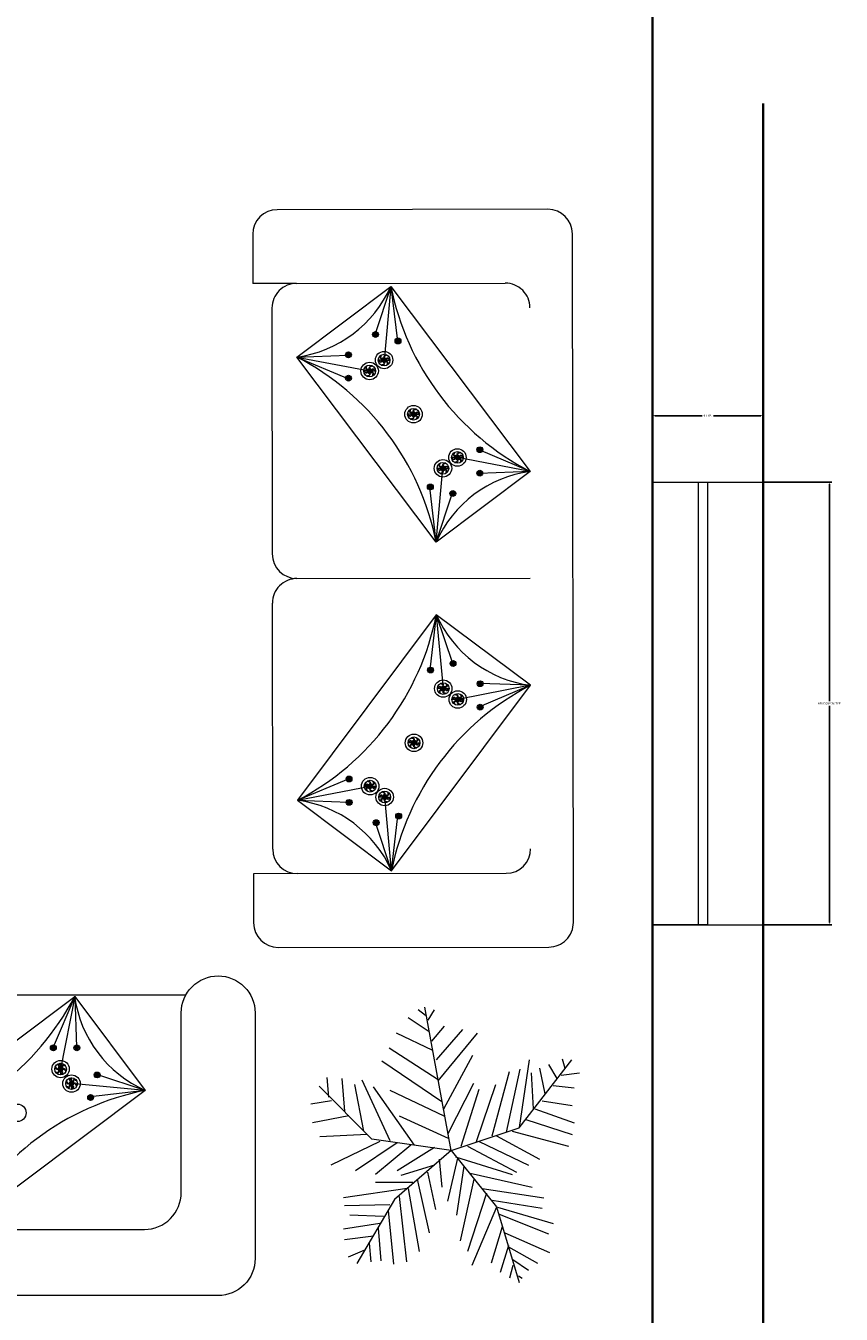
# Model space of a CAD drawing. Units: inches. Extents: x -61 to 1599, y -1316 to 257.
# Tile 199 of 204: x 1463 to 1529, y -166 to -61. Entities that reach past the tile are written whole.
import ezdxf

# ---------------------------------------------------------------- set-up
doc = ezdxf.new("R2010")
doc.units = ezdxf.units.IN
doc.header["$MEASUREMENT"] = 0
for name, color, linetype, lineweight in [('A-ANNO-DIMS', 2, 'Continuous', 18), ('FURNITURE', 83, 'Continuous', 18), ('WALLS', 4, 'Continuous', 35), ('WINDOWS', 220, 'Continuous', 18)]:
    doc.layers.add(name, color=color, linetype=linetype, lineweight=lineweight)
doc.layers.add('FUR', color=83, linetype='Continuous')
doc.styles.get("Standard").update_dxf_attribs({"font": 'arial.ttf'})
doc.dimstyles.get("Standard").update_dxf_attribs({"dimtxt": 0.18, "dimasz": 0.18, "dimexe": 0.18, "dimexo": 0.0625, "dimgap": 0.09, "dimtad": 0, "dimtih": 1, "dimtoh": 1, "dimdec": 0, "dimzin": 0, "dimdsep": 46, "dimlunit": 3, "dimtxsty": 'Standard', "dimcen": 0.09, "dimadec": 0, "dimazin": 0, "dimtfac": 1, "dimtdec": 0, "dimtofl": 0, "dimtmove": 0, "dimatfit": 3, "dimfxl": 1, "dimtolj": 1, "dimtzin": 0, "dimarcsym": 0})

# ---------------------------------------------------------------- blocks, each defined once
blk = doc.blocks.new('*U427')
at = {"layer": 'FUR'}
blk.add_open_spline([(0.01, 0.24), (-0.09, 0.14), (-0.29, -0.05), (0.22, -0.05), (0.07, -0.19), (0.01, -0.24)], degree=3, knots=[0, 0, 0, 0, 0.2846533, 0.5662105, 0.736751, 0.736751, 0.736751, 0.736751], dxfattribs=at)
blk = doc.blocks.new('*U428')
at = {"layer": 'FURNITURE', "transparency": 16777216}
for p, rotation in [((662.52, -238.49), 60), ((662.53, -238.73), 120), ((662.74, -238.83), 180), ((662.93, -238.46), 300), ((662.94, -238.7), 240)]:
    blk.add_blockref('*U427', p, dxfattribs=dict(at, rotation=rotation))
blk.add_blockref('*U427', (662.72, -238.36), dxfattribs=at)
blk = doc.blocks.new('*U441')
at = {"layer": 'FUR'}
blk.add_open_spline([(0.01, 0.24), (-0.09, 0.14), (-0.29, -0.05), (0.22, -0.05), (0.07, -0.19), (0.01, -0.24)], degree=3, knots=[0, 0, 0, 0, 0.2846533, 0.5662105, 0.736751, 0.736751, 0.736751, 0.736751], dxfattribs=at)
blk = doc.blocks.new('*U461')
at = {"layer": 'FURNITURE', "transparency": 16777216}
for p, rotation in [((662.52, -238.49), 60), ((662.53, -238.73), 120), ((662.74, -238.83), 180), ((662.93, -238.46), 300), ((662.94, -238.7), 240)]:
    blk.add_blockref('*U441', p, dxfattribs=dict(at, rotation=rotation))
blk.add_blockref('*U441', (662.72, -238.36), dxfattribs=at)
blk = doc.blocks.new('*U462')
at = {"layer": 'FUR'}
blk.add_open_spline([(0, 0.08), (-0.03, 0.05), (-0.1, -0.02), (0.08, -0.02), (0.02, -0.06), (0, -0.08)], degree=3, knots=[0, 0, 0, 0, 0.0954578, 0.1898773, 0.2470677, 0.2470677, 0.2470677, 0.2470677], dxfattribs=at)
blk = doc.blocks.new('*U463')
at = {"layer": 'FURNITURE', "transparency": 16777216}
for p, rotation in [((222.17, -79.98), 60), ((222.18, -80.06), 120), ((222.31, -79.97), 300), ((222.25, -80.09), 180), ((222.32, -80.05), 240)]:
    blk.add_blockref('*U462', p, dxfattribs=dict(at, rotation=rotation))
blk.add_blockref('*U462', (222.24, -79.93), dxfattribs=at)
blk = doc.blocks.new('*U429')
at = {"layer": 'FUR'}
blk.add_open_spline([(0, 0.08), (-0.03, 0.05), (-0.1, -0.02), (0.08, -0.02), (0.02, -0.06), (0, -0.08)], degree=3, knots=[0, 0, 0, 0, 0.0954578, 0.1898773, 0.2470677, 0.2470677, 0.2470677, 0.2470677], dxfattribs=at)
blk = doc.blocks.new('*U430')
at = {"layer": 'FURNITURE', "transparency": 16777216}
for p, rotation in [((222.17, -79.98), 60), ((222.18, -80.06), 120), ((222.31, -79.97), 300), ((222.25, -80.09), 180), ((222.32, -80.05), 240)]:
    blk.add_blockref('*U429', p, dxfattribs=dict(at, rotation=rotation))
blk.add_blockref('*U429', (222.24, -79.93), dxfattribs=at)
blk = doc.blocks.new('*U431')
at = {"layer": 'FUR'}
blk.add_open_spline([(0, 0.08), (-0.03, 0.05), (-0.1, -0.02), (0.08, -0.02), (0.02, -0.06), (0, -0.08)], degree=3, knots=[0, 0, 0, 0, 0.0954578, 0.1898773, 0.2470677, 0.2470677, 0.2470677, 0.2470677], dxfattribs=at)
blk = doc.blocks.new('*U432')
at = {"layer": 'FURNITURE', "transparency": 16777216}
for p, rotation in [((222.17, -79.98), 60), ((222.18, -80.06), 120), ((222.31, -79.97), 300), ((222.25, -80.09), 180), ((222.32, -80.05), 240)]:
    blk.add_blockref('*U431', p, dxfattribs=dict(at, rotation=rotation))
blk.add_blockref('*U431', (222.24, -79.93), dxfattribs=at)
blk = doc.blocks.new('*U433')
at = {"layer": 'FUR'}
blk.add_open_spline([(0, 0.08), (-0.03, 0.05), (-0.1, -0.02), (0.08, -0.02), (0.02, -0.06), (0, -0.08)], degree=3, knots=[0, 0, 0, 0, 0.0954578, 0.1898773, 0.2470677, 0.2470677, 0.2470677, 0.2470677], dxfattribs=at)
blk = doc.blocks.new('*U434')
at = {"layer": 'FURNITURE', "transparency": 16777216}
for p, rotation in [((222.17, -79.98), 60), ((222.18, -80.06), 120), ((222.31, -79.97), 300), ((222.25, -80.09), 180), ((222.32, -80.05), 240)]:
    blk.add_blockref('*U433', p, dxfattribs=dict(at, rotation=rotation))
blk.add_blockref('*U433', (222.24, -79.93), dxfattribs=at)
blk = doc.blocks.new('*U435')
at = {"layer": 'FUR'}
blk.add_open_spline([(0, 0.08), (-0.03, 0.05), (-0.1, -0.02), (0.08, -0.02), (0.02, -0.06), (0, -0.08)], degree=3, knots=[0, 0, 0, 0, 0.0954578, 0.1898773, 0.2470677, 0.2470677, 0.2470677, 0.2470677], dxfattribs=at)
blk = doc.blocks.new('*U436')
at = {"layer": 'FURNITURE', "transparency": 16777216}
for p, rotation in [((222.17, -79.98), 60), ((222.18, -80.06), 120), ((222.31, -79.97), 300), ((222.25, -80.09), 180), ((222.32, -80.05), 240)]:
    blk.add_blockref('*U435', p, dxfattribs=dict(at, rotation=rotation))
blk.add_blockref('*U435', (222.24, -79.93), dxfattribs=at)
blk = doc.blocks.new('*U437')
at = {"layer": 'FUR'}
blk.add_open_spline([(0, 0.08), (-0.03, 0.05), (-0.1, -0.02), (0.08, -0.02), (0.02, -0.06), (0, -0.08)], degree=3, knots=[0, 0, 0, 0, 0.0954578, 0.1898773, 0.2470677, 0.2470677, 0.2470677, 0.2470677], dxfattribs=at)
blk = doc.blocks.new('*U438')
at = {"layer": 'FURNITURE', "transparency": 16777216}
for p, rotation in [((222.17, -79.98), 60), ((222.18, -80.06), 120), ((222.31, -79.97), 300), ((222.25, -80.09), 180), ((222.32, -80.05), 240)]:
    blk.add_blockref('*U437', p, dxfattribs=dict(at, rotation=rotation))
blk.add_blockref('*U437', (222.24, -79.93), dxfattribs=at)
blk = doc.blocks.new('*U439')
at = {"layer": 'FUR'}
blk.add_open_spline([(0, 0.08), (-0.03, 0.05), (-0.1, -0.02), (0.08, -0.02), (0.02, -0.06), (0, -0.08)], degree=3, knots=[0, 0, 0, 0, 0.0954578, 0.1898773, 0.2470677, 0.2470677, 0.2470677, 0.2470677], dxfattribs=at)
blk = doc.blocks.new('*U465')
at = {"layer": 'FURNITURE', "transparency": 16777216}
for p, rotation in [((222.17, -79.98), 60), ((222.18, -80.06), 120), ((222.31, -79.97), 300), ((222.25, -80.09), 180), ((222.32, -80.05), 240)]:
    blk.add_blockref('*U439', p, dxfattribs=dict(at, rotation=rotation))
blk.add_blockref('*U439', (222.24, -79.93), dxfattribs=at)
blk = doc.blocks.new('*U466')
at = {"layer": 'FUR'}
blk.add_open_spline([(0, 0.08), (-0.03, 0.05), (-0.1, -0.02), (0.08, -0.02), (0.02, -0.06), (0, -0.08)], degree=3, knots=[0, 0, 0, 0, 0.0954578, 0.1898773, 0.2470677, 0.2470677, 0.2470677, 0.2470677], dxfattribs=at)
blk = doc.blocks.new('*U467')
at = {"layer": 'FURNITURE', "transparency": 16777216}
for p, rotation in [((222.17, -79.98), 60), ((222.18, -80.06), 120), ((222.31, -79.97), 300), ((222.25, -80.09), 180), ((222.32, -80.05), 240)]:
    blk.add_blockref('*U466', p, dxfattribs=dict(at, rotation=rotation))
blk.add_blockref('*U466', (222.24, -79.93), dxfattribs=at)
blk = doc.blocks.new('*U468')
at = {"layer": 'FUR'}
blk.add_open_spline([(0.01, 0.24), (-0.09, 0.14), (-0.29, -0.05), (0.22, -0.05), (0.07, -0.19), (0.01, -0.24)], degree=3, knots=[0, 0, 0, 0, 0.2846533, 0.5662105, 0.736751, 0.736751, 0.736751, 0.736751], dxfattribs=at)
blk = doc.blocks.new('*U469')
at = {"layer": 'FURNITURE', "transparency": 16777216}
for p, rotation in [((662.52, -238.49), 60), ((662.53, -238.73), 120), ((662.74, -238.83), 180), ((662.93, -238.46), 300), ((662.94, -238.7), 240)]:
    blk.add_blockref('*U468', p, dxfattribs=dict(at, rotation=rotation))
blk.add_blockref('*U468', (662.72, -238.36), dxfattribs=at)
blk = doc.blocks.new('*U470')
at = {"layer": 'FUR'}
blk.add_open_spline([(0.01, 0.24), (-0.09, 0.14), (-0.29, -0.05), (0.22, -0.05), (0.07, -0.19), (0.01, -0.24)], degree=3, knots=[0, 0, 0, 0, 0.2846533, 0.5662105, 0.736751, 0.736751, 0.736751, 0.736751], dxfattribs=at)
blk = doc.blocks.new('*U426')
at = {"layer": 'FURNITURE', "transparency": 16777216}
for p, rotation in [((662.52, -238.49), 60), ((662.53, -238.73), 120), ((662.74, -238.83), 180), ((662.93, -238.46), 300), ((662.94, -238.7), 240)]:
    blk.add_blockref('*U470', p, dxfattribs=dict(at, rotation=rotation))
blk.add_blockref('*U470', (662.72, -238.36), dxfattribs=at)
blk = doc.blocks.new('*U440')
at = {"layer": 'FUR'}
blk.add_open_spline([(0.01, 0.24), (-0.09, 0.14), (-0.29, -0.05), (0.22, -0.05), (0.07, -0.19), (0.01, -0.24)], degree=3, knots=[0, 0, 0, 0, 0.2846533, 0.5662105, 0.736751, 0.736751, 0.736751, 0.736751], dxfattribs=at)
blk = doc.blocks.new('*U464')
at = {"layer": 'FURNITURE', "transparency": 16777216}
for p, rotation in [((662.52, -238.49), 60), ((662.53, -238.73), 120), ((662.74, -238.83), 180), ((662.93, -238.46), 300), ((662.94, -238.7), 240)]:
    blk.add_blockref('*U440', p, dxfattribs=dict(at, rotation=rotation))
blk.add_blockref('*U440', (662.72, -238.36), dxfattribs=at)
blk = doc.blocks.new('*U423')
at = {"layer": 'FUR'}
blk.add_open_spline([(0.01, 0.24), (-0.09, 0.14), (-0.29, -0.05), (0.22, -0.05), (0.07, -0.19), (0.01, -0.24)], degree=3, knots=[0, 0, 0, 0, 0.2846533, 0.5662105, 0.736751, 0.736751, 0.736751, 0.736751], dxfattribs=at)
blk = doc.blocks.new('*U424')
at = {"layer": 'FURNITURE', "transparency": 16777216}
for p, rotation in [((662.52, -238.49), 60), ((662.53, -238.73), 120), ((662.74, -238.83), 180), ((662.93, -238.46), 300), ((662.94, -238.7), 240)]:
    blk.add_blockref('*U423', p, dxfattribs=dict(at, rotation=rotation))
blk.add_blockref('*U423', (662.72, -238.36), dxfattribs=at)
blk = doc.blocks.new('*U460')
at = {"layer": 'FUR'}
blk.add_open_spline([(0.01, 0.24), (-0.09, 0.14), (-0.29, -0.05), (0.22, -0.05), (0.07, -0.19), (0.01, -0.24)], degree=3, knots=[0, 0, 0, 0, 0.2846533, 0.5662105, 0.736751, 0.736751, 0.736751, 0.736751], dxfattribs=at)
blk = doc.blocks.new('*U442')
at = {"layer": 'FURNITURE', "transparency": 16777216}
for p, rotation in [((662.52, -238.49), 60), ((662.53, -238.73), 120), ((662.74, -238.83), 180), ((662.93, -238.46), 300), ((662.94, -238.7), 240)]:
    blk.add_blockref('*U460', p, dxfattribs=dict(at, rotation=rotation))
blk.add_blockref('*U460', (662.72, -238.36), dxfattribs=at)
blk = doc.blocks.new('*U443')
at = {"layer": 'FUR'}
blk.add_open_spline([(0, 0.08), (-0.03, 0.05), (-0.1, -0.02), (0.08, -0.02), (0.02, -0.06), (0, -0.08)], degree=3, knots=[0, 0, 0, 0, 0.0954578, 0.1898773, 0.2470677, 0.2470677, 0.2470677, 0.2470677], dxfattribs=at)
blk = doc.blocks.new('*U444')
at = {"layer": 'FURNITURE', "transparency": 16777216}
for p, rotation in [((222.17, -79.98), 60), ((222.18, -80.06), 120), ((222.31, -79.97), 300), ((222.25, -80.09), 180), ((222.32, -80.05), 240)]:
    blk.add_blockref('*U443', p, dxfattribs=dict(at, rotation=rotation))
blk.add_blockref('*U443', (222.24, -79.93), dxfattribs=at)
blk = doc.blocks.new('*U425')
at = {"layer": 'FUR'}
blk.add_open_spline([(0, 0.08), (-0.03, 0.05), (-0.1, -0.02), (0.08, -0.02), (0.02, -0.06), (0, -0.08)], degree=3, knots=[0, 0, 0, 0, 0.0954578, 0.1898773, 0.2470677, 0.2470677, 0.2470677, 0.2470677], dxfattribs=at)
blk = doc.blocks.new('*U449')
at = {"layer": 'FURNITURE', "transparency": 16777216}
for p, rotation in [((222.17, -79.98), 60), ((222.18, -80.06), 120), ((222.31, -79.97), 300), ((222.25, -80.09), 180), ((222.32, -80.05), 240)]:
    blk.add_blockref('*U425', p, dxfattribs=dict(at, rotation=rotation))
blk.add_blockref('*U425', (222.24, -79.93), dxfattribs=at)
blk = doc.blocks.new('*U450')
at = {"layer": 'FUR'}
blk.add_open_spline([(0, 0.08), (-0.03, 0.05), (-0.1, -0.02), (0.08, -0.02), (0.02, -0.06), (0, -0.08)], degree=3, knots=[0, 0, 0, 0, 0.0954578, 0.1898773, 0.2470677, 0.2470677, 0.2470677, 0.2470677], dxfattribs=at)
blk = doc.blocks.new('*U451')
at = {"layer": 'FURNITURE', "transparency": 16777216}
for p, rotation in [((222.17, -79.98), 60), ((222.18, -80.06), 120), ((222.31, -79.97), 300), ((222.25, -80.09), 180), ((222.32, -80.05), 240)]:
    blk.add_blockref('*U450', p, dxfattribs=dict(at, rotation=rotation))
blk.add_blockref('*U450', (222.24, -79.93), dxfattribs=at)
blk = doc.blocks.new('*U452')
at = {"layer": 'FUR'}
blk.add_open_spline([(0, 0.08), (-0.03, 0.05), (-0.1, -0.02), (0.08, -0.02), (0.02, -0.06), (0, -0.08)], degree=3, knots=[0, 0, 0, 0, 0.0954578, 0.1898773, 0.2470677, 0.2470677, 0.2470677, 0.2470677], dxfattribs=at)
blk = doc.blocks.new('*U453')
at = {"layer": 'FURNITURE', "transparency": 16777216}
for p, rotation in [((222.17, -79.98), 60), ((222.18, -80.06), 120), ((222.31, -79.97), 300), ((222.25, -80.09), 180), ((222.32, -80.05), 240)]:
    blk.add_blockref('*U452', p, dxfattribs=dict(at, rotation=rotation))
blk.add_blockref('*U452', (222.24, -79.93), dxfattribs=at)
blk = doc.blocks.new('*U454')
at = {"layer": 'FUR'}
blk.add_open_spline([(0, 0.08), (-0.03, 0.05), (-0.1, -0.02), (0.08, -0.02), (0.02, -0.06), (0, -0.08)], degree=3, knots=[0, 0, 0, 0, 0.0954578, 0.1898773, 0.2470677, 0.2470677, 0.2470677, 0.2470677], dxfattribs=at)
blk = doc.blocks.new('*U455')
at = {"layer": 'FURNITURE', "transparency": 16777216}
for p, rotation in [((222.17, -79.98), 60), ((222.18, -80.06), 120), ((222.31, -79.97), 300), ((222.25, -80.09), 180), ((222.32, -80.05), 240)]:
    blk.add_blockref('*U454', p, dxfattribs=dict(at, rotation=rotation))
blk.add_blockref('*U454', (222.24, -79.93), dxfattribs=at)
blk = doc.blocks.new('*U456')
at = {"layer": 'FUR'}
blk.add_open_spline([(0, 0.08), (-0.03, 0.05), (-0.1, -0.02), (0.08, -0.02), (0.02, -0.06), (0, -0.08)], degree=3, knots=[0, 0, 0, 0, 0.0954578, 0.1898773, 0.2470677, 0.2470677, 0.2470677, 0.2470677], dxfattribs=at)
blk = doc.blocks.new('*U457')
at = {"layer": 'FURNITURE', "transparency": 16777216}
for p, rotation in [((222.17, -79.98), 60), ((222.18, -80.06), 120), ((222.31, -79.97), 300), ((222.25, -80.09), 180), ((222.32, -80.05), 240)]:
    blk.add_blockref('*U456', p, dxfattribs=dict(at, rotation=rotation))
blk.add_blockref('*U456', (222.24, -79.93), dxfattribs=at)
blk = doc.blocks.new('*U458')
at = {"layer": 'FUR'}
blk.add_open_spline([(0, 0.08), (-0.03, 0.05), (-0.1, -0.02), (0.08, -0.02), (0.02, -0.06), (0, -0.08)], degree=3, knots=[0, 0, 0, 0, 0.0954578, 0.1898773, 0.2470677, 0.2470677, 0.2470677, 0.2470677], dxfattribs=at)
blk = doc.blocks.new('*U446')
at = {"layer": 'FURNITURE', "transparency": 16777216}
for p, rotation in [((222.17, -79.98), 60), ((222.18, -80.06), 120), ((222.31, -79.97), 300), ((222.25, -80.09), 180), ((222.32, -80.05), 240)]:
    blk.add_blockref('*U458', p, dxfattribs=dict(at, rotation=rotation))
blk.add_blockref('*U458', (222.24, -79.93), dxfattribs=at)
blk = doc.blocks.new('*U447')
at = {"layer": 'FUR'}
blk.add_open_spline([(0, 0.08), (-0.03, 0.05), (-0.1, -0.02), (0.08, -0.02), (0.02, -0.06), (0, -0.08)], degree=3, knots=[0, 0, 0, 0, 0.0954578, 0.1898773, 0.2470677, 0.2470677, 0.2470677, 0.2470677], dxfattribs=at)
blk = doc.blocks.new('*U448')
at = {"layer": 'FURNITURE', "transparency": 16777216}
for p, rotation in [((222.17, -79.98), 60), ((222.18, -80.06), 120), ((222.31, -79.97), 300), ((222.25, -80.09), 180), ((222.32, -80.05), 240)]:
    blk.add_blockref('*U447', p, dxfattribs=dict(at, rotation=rotation))
blk.add_blockref('*U447', (222.24, -79.93), dxfattribs=at)
blk = doc.blocks.new('*U419')
at = {"layer": 'FUR'}
blk.add_open_spline([(0.01, 0.24), (-0.09, 0.14), (-0.29, -0.05), (0.22, -0.05), (0.07, -0.19), (0.01, -0.24)], degree=3, knots=[0, 0, 0, 0, 0.2846533, 0.5662105, 0.736751, 0.736751, 0.736751, 0.736751], dxfattribs=at)
blk = doc.blocks.new('*U420')
at = {"layer": 'FURNITURE', "transparency": 16777216}
for p, rotation in [((662.52, -238.49), 60), ((662.53, -238.73), 120), ((662.74, -238.83), 180), ((662.93, -238.46), 300), ((662.94, -238.7), 240)]:
    blk.add_blockref('*U419', p, dxfattribs=dict(at, rotation=rotation))
blk.add_blockref('*U419', (662.72, -238.36), dxfattribs=at)
blk = doc.blocks.new('*U421')
at = {"layer": 'FUR'}
blk.add_open_spline([(0.01, 0.24), (-0.09, 0.14), (-0.29, -0.05), (0.22, -0.05), (0.07, -0.19), (0.01, -0.24)], degree=3, knots=[0, 0, 0, 0, 0.2846533, 0.5662105, 0.736751, 0.736751, 0.736751, 0.736751], dxfattribs=at)
blk = doc.blocks.new('*U422')
at = {"layer": 'FURNITURE', "transparency": 16777216}
for p, rotation in [((662.52, -238.49), 60), ((662.53, -238.73), 120), ((662.74, -238.83), 180), ((662.93, -238.46), 300), ((662.94, -238.7), 240)]:
    blk.add_blockref('*U421', p, dxfattribs=dict(at, rotation=rotation))
blk.add_blockref('*U421', (662.72, -238.36), dxfattribs=at)
blk = doc.blocks.new('*U459')
at = {"layer": 'FUR'}
blk.add_open_spline([(0.01, 0.24), (-0.09, 0.14), (-0.29, -0.05), (0.22, -0.05), (0.07, -0.19), (0.01, -0.24)], degree=3, knots=[0, 0, 0, 0, 0.2846533, 0.5662105, 0.736751, 0.736751, 0.736751, 0.736751], dxfattribs=at)
blk = doc.blocks.new('*U445')
at = {"layer": 'FURNITURE', "transparency": 16777216}
for p, rotation in [((662.52, -238.49), 60), ((662.53, -238.73), 120), ((662.74, -238.83), 180), ((662.93, -238.46), 300), ((662.94, -238.7), 240)]:
    blk.add_blockref('*U459', p, dxfattribs=dict(at, rotation=rotation))
blk.add_blockref('*U459', (662.72, -238.36), dxfattribs=at)
blk = doc.blocks.new('*U264')
for p, q in [((0, 0), (-10.5, 57)), ((-8.737, 47.138), (-17.069, 52.711)), ((-10.186, 53.64), (-13.084, 55.962)), ((-9.099, 51.782), (-6.563, 55.962)), ((-7.288, 39.707), (-21.778, 46.673)), ((-7.65, 43.423), (-2.578, 49.46)), ((-5.839, 35.992), (4.667, 48.067)), ((-5.114, 27.632), (10.463, 46.673)), ((-5.114, 28.097), (-24.676, 40.636)), ((-2.941, 16.486), (8.652, 37.85)), ((27, 9), (48, 36)), ((27.127, 9.056), (31.112, 35.992)), ((44.153, 36.456), (45.239, 32.741)), ((-3.665, 19.273), (-27.574, 35.527)), ((16.259, 5.805), (23.142, 31.348)), ((22.055, 7.198), (27.489, 32.277)), ((31.836, 30.883), (32.561, 16.486)), ((35.096, 32.741), (37.27, 22.524)), ((38.719, 34.134), (41.979, 28.561)), ((43.791, 29.954), (51.036, 30.883)), ((-48.585, 21.131), (-49.309, 29.026)), ((-43.513, 28.561), (-42.427, 15.558)), ((-38.442, 26.239), (-34.819, 7.663)), ((-35.544, 28.097), (-24.314, 3.947)), ((-1.129, 6.734), (9.014, 26.704)), ((10.101, 3.483), (17.708, 26.239)), ((40.53, 25.775), (48.862, 24.846)), ((-31.5, 4.5), (-52.5, 25.5)), ((-14.533, 2.09), (-30.834, 25.31)), ((-24.314, 23.917), (-2.941, 13.7)), ((3.942, 1.625), (11.187, 24.381)), ((-47.498, 19.737), (-55.83, 18.344)), ((33.285, 16.486), (48.862, 10.913)), ((36.183, 19.737), (48.137, 17.88)), ((-40.615, 13.7), (-55.105, 10.913)), ((-20.691, 13.7), (-1.129, 4.876)), ((29.662, 12.307), (48.137, 6.269)), ((-33.37, 6.269), (-52.207, 5.34)), ((0, 0), (27, 9)), ((18.07, 5.805), (35.096, -3.483)), ((24.229, 7.663), (46.688, 1.625)), ((-28.299, 3.483), (-47.86, -5.805)), ((-21.416, 3.018), (-38.079, -8.128)), ((0, 0), (-31.5, 4.5)), ((-15.982, 2.09), (-30.11, -9.521)), ((0, 0), (-22.5, -19.5)), ((-6.563, 1.161), (-21.416, -8.128)), ((0, 0), (18, -22.5)), ((6.478, 1.625), (26.04, -8.592)), ((11.187, 3.483), (30.749, -5.805)), ((-4.752, -3.483), (-3.665, -14.629)), ((2.493, -3.019), (-1.491, -20.202)), ((1.769, -2.555), (24.229, -9.521)), ((-6.563, -5.805), (-19.967, -9.985)), ((-9.461, -8.592), (-6.201, -23.453)), ((5.029, -6.27), (2.131, -25.775)), ((7.565, -9.056), (32.198, -14.629)), ((-17.431, -15.094), (-42.789, -18.809)), ((-15.257, -12.772), (-30.11, -12.772)), ((-17.069, -15.094), (-12.721, -40.172)), ((-13.446, -11.378), (-8.737, -32.741)), ((9.014, -11.378), (3.58, -35.992)), ((12.274, -15.094), (36.907, -18.809)), ((-22.5, -19.5), (-37.5, -45)), ((-20.691, -18.345), (-17.793, -44.352)), ((14.085, -16.951), (6.478, -40.172)), ((16.259, -19.738), (36.183, -22.989)), ((-24.314, -21.596), (-42.427, -22.06)), ((-25.038, -23.918), (-22.865, -45.281)), ((18.07, -22.524), (8.289, -45.745)), ((18, -22.5), (27, -52.5)), ((18.433, -22.524), (40.53, -29.026)), ((19.157, -25.311), (38.719, -33.206)), ((-28.299, -29.026), (-42.789, -31.348)), ((-26.849, -26.24), (-40.253, -25.775)), ((20.244, -30.419), (15.897, -44.816)), ((-30.834, -34.135), (-42.427, -35.528)), ((-29.023, -30.884), (-27.936, -43.887)), ((21.331, -32.741), (39.081, -40.636)), ((-34.457, -39.708), (-40.978, -42.494)), ((-32.646, -36.921), (-31.921, -44.352)), ((22.78, -37.85), (19.519, -48.532)), ((22.78, -38.314), (34.372, -44.816)), ((24.591, -45.745), (23.142, -50.854)), ((24.591, -43.423), (30.749, -47.603)), ((26.764, -49.925), (28.213, -50.854))]:
    blk.add_line(p, q)
blk = doc.blocks.new('WIN-36IN')
for p, q in [((0, 4.5), (0, 9)), ((0, 9), (0, 0)), ((36, 9), (36, 0)), ((0, 5.26), (36, 5.26)), ((0, 4.5), (36, 4.5)), ((0, 4.5), (36, 4.5))]:
    blk.add_line(p, q)
blk = doc.blocks.new('*U120')
at = {"layer": 'FUR'}
blk.add_open_spline([(0, 0.08), (-0.03, 0.05), (-0.1, -0.02), (0.08, -0.02), (0.02, -0.06), (0, -0.08)], degree=3, knots=[0, 0, 0, 0, 0.0954578, 0.1898773, 0.2470677, 0.2470677, 0.2470677, 0.2470677], dxfattribs=at)
blk = doc.blocks.new('*U121')
at = {"layer": 'FUR', "transparency": 16777216}
for p, rotation in [((222.17, -79.98), 60), ((222.18, -80.06), 120), ((222.31, -79.97), 300), ((222.25, -80.09), 180), ((222.32, -80.05), 240)]:
    blk.add_blockref('*U120', p, dxfattribs=dict(at, rotation=rotation))
blk.add_blockref('*U120', (222.24, -79.93), dxfattribs=at)
blk = doc.blocks.new('*U140')
at = {"layer": 'FUR'}
blk.add_open_spline([(0.01, 0.24), (-0.09, 0.14), (-0.29, -0.05), (0.22, -0.05), (0.07, -0.19), (0.01, -0.24)], degree=3, knots=[0, 0, 0, 0, 0.2846533, 0.5662105, 0.736751, 0.736751, 0.736751, 0.736751], dxfattribs=at)
blk = doc.blocks.new('*U141')
at = {"layer": 'FUR', "transparency": 16777216}
for p, rotation in [((662.52, -238.49), 60), ((662.53, -238.73), 120), ((662.74, -238.83), 180), ((662.93, -238.46), 300), ((662.94, -238.7), 240)]:
    blk.add_blockref('*U140', p, dxfattribs=dict(at, rotation=rotation))
blk.add_blockref('*U140', (662.72, -238.36), dxfattribs=at)
blk = doc.blocks.new('*U135')
at = {"layer": 'FUR'}
blk.add_open_spline([(0.01, 0.24), (-0.09, 0.14), (-0.29, -0.05), (0.22, -0.05), (0.07, -0.19), (0.01, -0.24)], degree=3, knots=[0, 0, 0, 0, 0.2846533, 0.5662105, 0.736751, 0.736751, 0.736751, 0.736751], dxfattribs=at)
blk = doc.blocks.new('*U136')
at = {"layer": 'FUR', "transparency": 16777216}
for p, rotation in [((662.52, -238.49), 60), ((662.53, -238.73), 120), ((662.74, -238.83), 180), ((662.93, -238.46), 300), ((662.94, -238.7), 240)]:
    blk.add_blockref('*U135', p, dxfattribs=dict(at, rotation=rotation))
blk.add_blockref('*U135', (662.72, -238.36), dxfattribs=at)
blk = doc.blocks.new('*U118')
at = {"layer": 'FUR'}
blk.add_open_spline([(0, 0.08), (-0.03, 0.05), (-0.1, -0.02), (0.08, -0.02), (0.02, -0.06), (0, -0.08)], degree=3, knots=[0, 0, 0, 0, 0.0954578, 0.1898773, 0.2470677, 0.2470677, 0.2470677, 0.2470677], dxfattribs=at)
blk = doc.blocks.new('*U119')
at = {"layer": 'FUR', "transparency": 16777216}
for p, rotation in [((222.17, -79.98), 60), ((222.18, -80.06), 120), ((222.31, -79.97), 300), ((222.25, -80.09), 180), ((222.32, -80.05), 240)]:
    blk.add_blockref('*U118', p, dxfattribs=dict(at, rotation=rotation))
blk.add_blockref('*U118', (222.24, -79.93), dxfattribs=at)
blk = doc.blocks.new('*U138')
at = {"layer": 'FUR'}
blk.add_open_spline([(0, 0.08), (-0.03, 0.05), (-0.1, -0.02), (0.08, -0.02), (0.02, -0.06), (0, -0.08)], degree=3, knots=[0, 0, 0, 0, 0.0954578, 0.1898773, 0.2470677, 0.2470677, 0.2470677, 0.2470677], dxfattribs=at)
blk = doc.blocks.new('*U139')
at = {"layer": 'FUR', "transparency": 16777216}
for p, rotation in [((222.17, -79.98), 60), ((222.18, -80.06), 120), ((222.31, -79.97), 300), ((222.25, -80.09), 180), ((222.32, -80.05), 240)]:
    blk.add_blockref('*U138', p, dxfattribs=dict(at, rotation=rotation))
blk.add_blockref('*U138', (222.24, -79.93), dxfattribs=at)
blk = doc.blocks.new('*U122')
at = {"layer": 'FUR'}
blk.add_open_spline([(0, 0.08), (-0.03, 0.05), (-0.1, -0.02), (0.08, -0.02), (0.02, -0.06), (0, -0.08)], degree=3, knots=[0, 0, 0, 0, 0.0954578, 0.1898773, 0.2470677, 0.2470677, 0.2470677, 0.2470677], dxfattribs=at)
blk = doc.blocks.new('*U137')
at = {"layer": 'FUR', "transparency": 16777216}
for p, rotation in [((222.17, -79.98), 60), ((222.18, -80.06), 120), ((222.31, -79.97), 300), ((222.25, -80.09), 180), ((222.32, -80.05), 240)]:
    blk.add_blockref('*U122', p, dxfattribs=dict(at, rotation=rotation))
blk.add_blockref('*U122', (222.24, -79.93), dxfattribs=at)
blk = doc.blocks.new('SOFA-THREE-SEAT')
for p, q in [((78.37, 24.44), (57, 24.44)), ((69.34, 24.33), (67.59, 20.19)), ((69.34, 24.33), (68.19, 18.42)), ((69.34, 24.33), (69.49, 20.19)), ((67.6, 20.14), (67.6, 20.3)), ((67.6, 20.14), (67.6, 19.98)), ((69.51, 20.14), (69.51, 20.3)), ((69.51, 20.14), (69.51, 19.98)), ((68.19, 18.42), (68.19, 18.9)), ((68.19, 18.42), (68.19, 17.95)), ((75.07, 16.69), (71.14, 17.99)), ((71.16, 17.94), (71.16, 18.1)), ((71.16, 17.94), (71.16, 17.78)), ((69.08, 17.24), (69.08, 17.72)), ((75.07, 16.69), (69.08, 17.24)), ((69.08, 17.24), (69.08, 16.77)), ((75.07, 16.69), (70.61, 16.16)), ((70.63, 16.11), (70.63, 16.27)), ((70.63, 16.11), (70.63, 15.95))]:
    blk.add_line(p, q)
blk.add_lwpolyline([(78, 8.38), (78, 23, -0.414214), (81, 26), (81, 26, -0.414214), (84, 23), (84, 3, -0.414214), (81, 0), (3, 0, -0.414214), (0, 3), (0, 23, -0.414214), (3, 26), (3, 26, -0.414214), (6, 23), (6, 8.38, 0.414214), (9, 5.38), (75, 5.38, 0.414214)], format="xyb", close=True)
blk.add_lwpolyline([(54.27, 13.03), (69.34, 24.33), (75.07, 16.69), (60.01, 5.38)], close=True)
for centre, radius in [((67.6, 20.14), 0.238), ((67.6, 20.14), 0.16), ((69.51, 20.14), 0.238), ((69.51, 20.14), 0.16), ((68.19, 18.42), 0.71), ((68.19, 18.42), 0.476), ((69.08, 17.24), 0.71), ((71.16, 17.94), 0.238), ((71.16, 17.94), 0.16), ((69.08, 17.24), 0.476), ((70.63, 16.11), 0.238), ((70.63, 16.11), 0.16), ((64.67, 14.86), 0.71)]:
    blk.add_circle(centre, radius)
for centre, radius, start, end in [((50.05, 34.34), 21.73, 281.2044, 332.5684), ((79.06, 25.66), 9.82, 187.747, 246.0258), ((79.3, -4.63), 21.73, 101.2044, 152.5684)]:
    blk.add_arc(centre, radius, start, end)
at = {"rotation": 180}
for name, p in [('*U121', (289.85, -59.87)), ('*U119', (291.75, -59.87)), ('*U141', (730.92, -220.17)), ('*U137', (293.4, -62.07)), ('*U136', (731.81, -221.35)), ('*U139', (292.87, -63.9))]:
    blk.add_blockref(name, p, dxfattribs=at)
blk = doc.blocks.new('*D618')
at = {"layer": 'A-ANNO-DIMS', "color": 0, "lineweight": -2, "transparency": 16777216}
for p, q in [((1522.77, -97.97), (1528.28, -97.97)), ((1528.1, -98.15), (1528.1, -115.79)), ((1528.1, -133.79), (1528.1, -116.16)), ((1522.77, -133.97), (1528.28, -133.97))]:
    blk.add_line(p, q, dxfattribs=at)
at = {"layer": 'A-ANNO-DIMS', "color": 0, "transparency": 16777216}
for points in [[(1528.07, -98.15), (1528.13, -98.15), (1528.1, -97.97)], [(1528.07, -133.79), (1528.13, -133.79), (1528.1, -133.97)]]:
    blk.add_solid(points, dxfattribs=at)
at = {"layer": 'DEFPOINTS', "color": 0, "transparency": 16777216}
for p in [(1522.7, -97.97), (1528.1, -97.97), (1522.7, -133.97)]:
    blk.add_point(p, dxfattribs=at)
at = {"layer": 'A-ANNO-DIMS', "color": 0, "transparency": 16777216, "insert": (1528.1, -115.97), "char_height": 0.18, "attachment_point": 5}
blk.add_mtext('\\A1;WINDOW 36 TYP.', dxfattribs=at)
blk = doc.blocks.new('*D619')
at = {"layer": 'A-ANNO-DIMS', "color": 0, "lineweight": -2, "transparency": 16777216}
for p, q in [((1513.7, -97.91), (1513.7, -92.39)), ((1513.88, -92.57), (1517.74, -92.57)), ((1522.52, -92.57), (1518.66, -92.57)), ((1522.7, -97.91), (1522.7, -92.39))]:
    blk.add_line(p, q, dxfattribs=at)
at = {"layer": 'A-ANNO-DIMS', "color": 0, "transparency": 16777216}
for points in [[(1513.88, -92.54), (1513.88, -92.6), (1513.7, -92.57)], [(1522.52, -92.54), (1522.52, -92.6), (1522.7, -92.57)]]:
    blk.add_solid(points, dxfattribs=at)
at = {"layer": 'DEFPOINTS', "color": 0, "transparency": 16777216}
for p in [(1513.7, -92.57), (1513.7, -97.97), (1522.7, -97.97)]:
    blk.add_point(p, dxfattribs=at)
at = {"layer": 'A-ANNO-DIMS', "color": 0, "transparency": 16777216, "insert": (1518.2, -92.57), "char_height": 0.18, "attachment_point": 5}
blk.add_mtext('\\A1;9 TYP.', dxfattribs=at)

msp = doc.modelspace()

# ---------------------------------------------------------------- linework, layer by layer
at = {"layer": 'FURNITURE'}
for p, q in [((1484.7579, -81.8149), (1481.1999, -81.8197)), ((1484.7579, -81.8149), (1501.7299, -81.7915)), ((1492.4247, -82.0531), (1491.1247, -85.9885)), ((1492.4247, -82.0531), (1491.8773, -88.0479)), ((1492.4247, -82.0531), (1492.9538, -86.5181)), ((1482.7607, -83.8176), (1482.7882, -103.8176)), ((1491.1772, -85.9691), (1491.0174, -85.9693)), ((1491.1772, -85.9691), (1491.337, -85.9689)), ((1493.0062, -86.4987), (1492.8464, -86.4989)), ((1493.0062, -86.4987), (1493.166, -86.4984)), ((1484.7866, -87.8015), (1488.9281, -87.6417)), ((1484.7866, -87.8015), (1490.6987, -88.9349)), ((1484.7866, -87.8015), (1488.9307, -89.5458)), ((1488.9805, -87.6223), (1488.8207, -87.6225)), ((1488.9805, -87.6223), (1489.1403, -87.6221)), ((1490.6987, -88.9349), (1490.2222, -88.9356)), ((1490.6987, -88.9349), (1491.1752, -88.9342)), ((1491.8773, -88.0479), (1491.4008, -88.0485)), ((1491.8773, -88.0479), (1492.3538, -88.0472)), ((1488.9831, -89.5264), (1488.8233, -89.5266)), ((1488.9831, -89.5264), (1489.1429, -89.5262)), ((1494.2688, -92.452), (1493.7923, -92.4527)), ((1494.2688, -92.452), (1494.7452, -92.4514)), ((1499.6593, -95.3388), (1499.4995, -95.339)), ((1503.7509, -97.1025), (1499.6068, -95.3582)), ((1499.6593, -95.3388), (1499.8191, -95.3385)), ((1497.8388, -95.9691), (1497.3623, -95.9698)), ((1497.8388, -95.9691), (1498.3153, -95.9685)), ((1503.7509, -97.1025), (1497.8388, -95.9691)), ((1496.1128, -102.851), (1496.6602, -96.8562)), ((1496.6602, -96.8562), (1496.1837, -96.8568)), ((1496.6602, -96.8562), (1497.1367, -96.8555)), ((1499.6619, -97.2429), (1499.5021, -97.2431)), ((1503.7509, -97.1025), (1499.6094, -97.2623)), ((1499.6619, -97.2429), (1499.8217, -97.2427)), ((1495.6362, -98.3665), (1495.4764, -98.3667)), ((1496.1128, -102.851), (1495.5838, -98.386)), ((1495.6362, -98.3665), (1495.796, -98.3663)), ((1496.1128, -102.851), (1497.4128, -98.9155)), ((1497.4652, -98.8961), (1497.3054, -98.8963)), ((1497.4652, -98.8961), (1497.625, -98.8959)), ((1484.7909, -105.8149), (1503.7629, -105.7888)), ((1484.7909, -105.8149), (1484.7909, -105.8149)), ((1482.8212, -127.8176), (1482.7937, -107.8176)), ((1496.121, -108.7733), (1495.6042, -113.2397)), ((1496.121, -108.7733), (1496.6848, -114.7666)), ((1496.121, -108.7733), (1497.4317, -112.7051)), ((1497.4842, -112.7244), (1497.3244, -112.7246)), ((1497.4842, -112.7244), (1497.644, -112.7242)), ((1495.6567, -113.259), (1495.4969, -113.2592)), ((1495.6567, -113.259), (1495.8165, -113.2588)), ((1496.6848, -114.7666), (1496.2084, -114.7672)), ((1496.6848, -114.7666), (1497.1613, -114.7659)), ((1503.7748, -114.5007), (1497.8659, -115.6503)), ((1499.6854, -114.3716), (1499.5256, -114.3718)), ((1503.7748, -114.5007), (1499.6329, -114.3523)), ((1503.7748, -114.5007), (1499.6355, -116.2564)), ((1499.6854, -114.3716), (1499.8452, -114.3713)), ((1497.8659, -115.6503), (1497.3894, -115.651)), ((1497.8659, -115.6503), (1498.3424, -115.6497)), ((1499.688, -116.2757), (1499.5283, -116.2759)), ((1499.688, -116.2757), (1499.8478, -116.2755)), ((1494.3055, -119.1773), (1493.829, -119.1779)), ((1494.3055, -119.1773), (1494.782, -119.1766)), ((1484.8361, -123.8538), (1488.9754, -122.0981)), ((1489.0279, -122.1174), (1488.8681, -122.1176)), ((1489.0279, -122.1174), (1489.1877, -122.1172)), ((1484.8361, -123.8538), (1490.7451, -122.7042)), ((1490.7451, -122.7042), (1490.2686, -122.7048)), ((1490.7451, -122.7042), (1491.2216, -122.7035)), ((1491.9261, -123.588), (1491.4496, -123.5886)), ((1491.9261, -123.588), (1492.4026, -123.5873)), ((1492.49, -129.5812), (1491.9261, -123.588)), ((1484.8361, -123.8538), (1488.978, -124.0022)), ((1489.0305, -124.0215), (1488.8708, -124.0217)), ((1489.0305, -124.0215), (1489.1903, -124.0213)), ((1491.2318, -125.6687), (1491.072, -125.6689)), ((1492.49, -129.5812), (1491.1793, -125.6494)), ((1491.2318, -125.6687), (1491.3915, -125.6685)), ((1492.49, -129.5812), (1493.0068, -125.1148)), ((1493.0593, -125.1341), (1492.8995, -125.1343)), ((1493.0593, -125.1341), (1493.2191, -125.1338)), ((1484.8239, -129.8148), (1481.2659, -129.8197)), ((1484.8239, -129.8148), (1501.7958, -129.7915))]:
    msp.add_line(p, q, dxfattribs=at)
msp.add_lwpolyline([(1481.2659, -129.8197), (1481.2714, -133.8197, 0.41421356), (1483.2742, -135.817), (1505.2741, -135.7867, 0.41421369), (1507.2714, -133.784), (1507.1944, -77.784, 0.41421343), (1505.1916, -75.7868), (1483.1917, -75.817, 0.41421356), (1481.1944, -77.8197), (1481.1999, -81.8197)], format="xyb", dxfattribs=at)
for points in [[(1496.1128, -102.851), (1484.7866, -87.8015), (1492.4247, -82.0531), (1503.7509, -97.1025)], [(1496.121, -108.7733), (1484.8361, -123.8538), (1492.49, -129.5812), (1503.7748, -114.5007)]]:
    msp.add_lwpolyline(points, close=True, dxfattribs=at)
for centre, radius in [((1491.1772, -85.9691), 0.2382), ((1491.1772, -85.9691), 0.1598), ((1493.0062, -86.4987), 0.2382), ((1493.0062, -86.4987), 0.1598), ((1488.9805, -87.6223), 0.2382), ((1488.9805, -87.6223), 0.1598), ((1491.8773, -88.0479), 0.7104), ((1491.8773, -88.0479), 0.4765), ((1490.6987, -88.9349), 0.7104), ((1490.6987, -88.9349), 0.4765), ((1488.9831, -89.5264), 0.2382), ((1488.9831, -89.5264), 0.1598), ((1494.2688, -92.452), 0.7104), ((1494.2688, -92.452), 0.4765), ((1497.8388, -95.9691), 0.7104), ((1499.6593, -95.3388), 0.2382), ((1499.6593, -95.3388), 0.1598), ((1496.6602, -96.8562), 0.7104), ((1496.6602, -96.8562), 0.4765), ((1497.8388, -95.9691), 0.4765), ((1499.6619, -97.2429), 0.2382), ((1499.6619, -97.2429), 0.1598), ((1495.6362, -98.3665), 0.2382), ((1495.6362, -98.3665), 0.1598), ((1497.4652, -98.8961), 0.2382), ((1497.4652, -98.8961), 0.1598), ((1495.6567, -113.259), 0.2382), ((1495.6567, -113.259), 0.1598), ((1497.4842, -112.7244), 0.2382), ((1497.4842, -112.7244), 0.1598), ((1496.6848, -114.7666), 0.7104), ((1499.6854, -114.3716), 0.2382), ((1499.6854, -114.3716), 0.1598), ((1496.6848, -114.7666), 0.4765), ((1497.8659, -115.6503), 0.7104), ((1497.8659, -115.6503), 0.4765), ((1499.688, -116.2757), 0.2382), ((1499.688, -116.2757), 0.1598), ((1494.3055, -119.1773), 0.7104), ((1494.3055, -119.1773), 0.4765), ((1489.0279, -122.1174), 0.2382), ((1489.0279, -122.1174), 0.1598), ((1490.7451, -122.7042), 0.7104), ((1490.7451, -122.7042), 0.4765), ((1491.9261, -123.588), 0.7104), ((1491.9261, -123.588), 0.4765), ((1489.0305, -124.0215), 0.2382), ((1489.0305, -124.0215), 0.1598), ((1491.2318, -125.6687), 0.2382), ((1491.2318, -125.6687), 0.1598), ((1493.0593, -125.1341), 0.2382), ((1493.0593, -125.1341), 0.1598)]:
    msp.add_circle(centre, radius, dxfattribs=at)
for centre, radius, start, end in [((1484.7607, -83.8148), 2, 90.078764, 180.078764), ((1483.45, -78.0769), 9.816, 277.825767, 336.104516), ((1513.7357, -77.8012), 21.731, 191.283178, 242.647105), ((1501.7326, -83.7915), 2, 0.078749, 90.078764), ((1474.8019, -107.1028), 21.731, 11.283178, 62.647105), ((1505.0875, -106.8271), 9.816, 97.825767, 156.104516), ((1484.7882, -103.8149), 2, 180.078764, 270.078764), ((1484.7937, -107.8149), 2, 90.078764, 180.078764), ((1474.7984, -104.58), 21.731, 297.510392, 348.87432), ((1505.0847, -104.7725), 9.816, 204.052981, 262.33173), ((1513.8126, -133.7745), 21.731, 117.510392, 168.87432), ((1483.5263, -133.5821), 9.816, 24.052981, 82.33173), ((1484.8212, -127.8148), 2, 180.078764, 270.078764), ((1501.7931, -127.7915), 2, 270.078764, 0.078749)]:
    msp.add_arc(centre, radius, start, end, dxfattribs=at)
at = {"layer": 'WALLS'}
for p, q in [((1513.7028, -13.3229), (1513.7028, -175.3229)), ((1522.7028, -441.3229), (1522.7028, -67.169))]:
    msp.add_line(p, q, dxfattribs=at)

# ---------------------------------------------------------------- block references
at = {"layer": 'FURNITURE', "rotation": 270.0787336990067}
for name, p in [('*U446', (1570.884, 136.3856)), ('*U448', (1572.713, 135.856)), ('*U455', (1568.6874, 134.7324)), ('*U445', (1729.5615, 575.0095)), ('*U420', (1728.383, 574.1225)), ('*U457', (1568.69, 132.8283)), ('*U424', (1731.953, 570.6054)), ('*U444', (1579.3661, 127.0159)), ('*U422', (1734.3445, 566.2012)), ('*U442', (1735.5231, 567.0882)), ('*U449', (1579.3687, 125.1118)), ('*U453', (1575.343, 123.9882)), ('*U451', (1577.1721, 123.4586))]:
    msp.add_blockref(name, p, dxfattribs=at)
at = {"layer": 'FURNITURE', "xscale": -1, "rotation": 270.0787636990076}
for name, p in [('*U434', (1575.9744, -335.3938)), ('*U432', (1577.802, -334.8591)), ('*U430', (1580.0032, -336.5063)), ('*U426', (1736.1909, -777.1681)), ('*U461', (1737.3719, -778.0518)), ('*U463', (1580.0058, -338.4105)), ('*U428', (1733.8115, -781.5788)), ('*U438', (1569.3457, -344.2521)), ('*U469', (1730.2511, -785.1057)), ('*U464', (1731.4321, -785.9895)), ('*U436', (1569.3483, -346.1563)), ('*U465', (1571.5495, -347.8034)), ('*U467', (1573.3771, -347.2688))]:
    msp.add_blockref(name, p, dxfattribs=at)
at = {"layer": 'FURNITURE'}
msp.add_blockref('SOFA-THREE-SEAT', (1397.3851, -164.1303), dxfattribs=at)
at = {"layer": 'FURNITURE', "xscale": 0.2045054661246738, "yscale": 0.2045054661246738, "zscale": 0.2045054661246738}
msp.add_blockref('*U264', (1497.3277, -152.3267), dxfattribs=at)
at = {"layer": 'WINDOWS', "rotation": 89.99999999999982}
msp.add_blockref('WIN-36IN', (1522.7029, -133.972), dxfattribs=at)

# ---------------------------------------------------------------- dimensions: what is measured, and where the dimension line sits
at = {"layer": 'A-ANNO-DIMS'}
for base, p1, p2, angle, text, picture, middle in [((1513.7028, -92.5719), (1522.7028, -97.9719), (1513.7028, -97.9719), 180, '<> TYP.', '*D619', (1518.2028, -92.5719)), ((1528.1028, -97.9719), (1522.7028, -133.9719), (1522.7028, -97.9719), 90, 'WINDOW <> TYP.', '*D618', (1528.1028, -115.9719))]:
    dim = msp.add_linear_dim(base=base, p1=p1, p2=p2, angle=angle, text=text, dimstyle='Standard', override={"dimdec": 0, "dimlfac": 1, "dimrnd": 0, "dimzin": 0, "dimdsep": 46, "dimlunit": 2}, dxfattribs=at)
    dim.commit()
    dim.dimension.update_dxf_attribs({"geometry": picture, "text_midpoint": middle})

doc.saveas('drawing.dxf')
